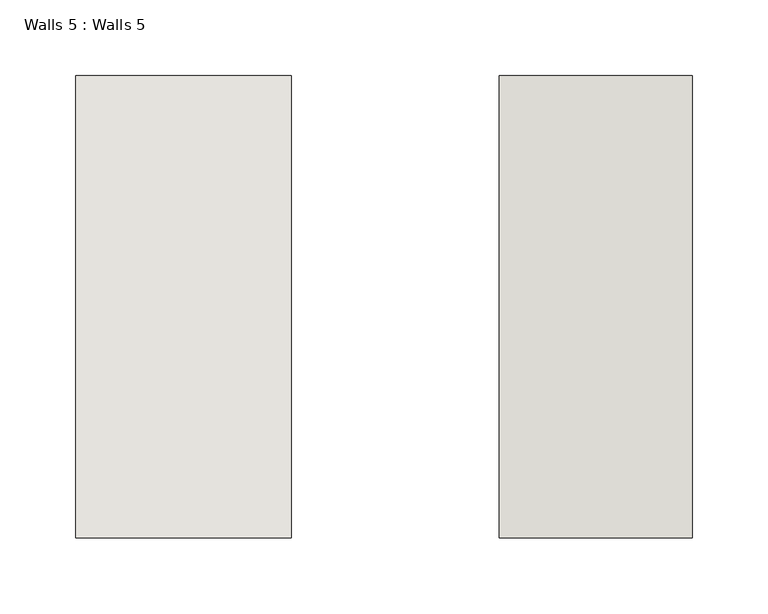
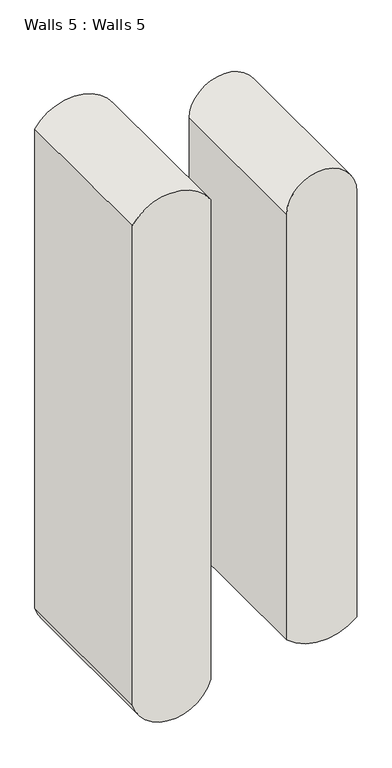
"""IFC4 building model written with IfcOpenShell, lengths in millimetres: wall geometry, Walls 5 : Walls 5."""

from ifc_helpers import new_model, si_unit, point, frame, frame_2d, origin, place, context, project, spatial, polyline, circle_curve, trimmed, segment, composite_curve, outline, extrude, source, transform, mapped, element, save


def walls_5_walls_5_0e8582f5(model_context):
    return source(origin(), model_context, "Body", "SweptSolid", [
        extrude(outline(composite_curve([segment(polyline([(1044.1671837, -3357.2945035), (127.0, -3357.2945035)]), True, "CONTINUOUS"), segment(trimmed(circle_curve(frame_2d((147.9342511, -3286.3689154)), 73.950537), [point((127.0, -3357.2945035))], [point((127.0, -3215.4433272))], False, "CARTESIAN"), True, "CONTINUOUS"), segment(polyline([(127.0, -3215.4433272), (1044.1671837, -3215.4433272)]), True, "CONTINUOUS"), segment(trimmed(circle_curve(frame_2d((996.2397239, -3286.3689154)), 85.6007036), [point((1044.1671837, -3215.4433272))], [point((1044.1671837, -3357.2945035))], False, "CARTESIAN"), True, "CONTINUOUS")], self_intersect=False)), frame((0.0, -3748.3510925, 0.0), z_axis=(0.0, 1.0, 0.0), x_axis=(0.0, 0.0, 1.0)), (0.0, 0.0, 1.0), 304.8),
        extrude(outline(composite_curve([segment(polyline([(966.6038696, -3078.1550887), (153.8038696, -3078.1550887)]), True, "CONTINUOUS"), segment(trimmed(circle_curve(frame_2d((225.1761374, -3014.6550887)), 95.5314116), [point((153.8038696, -3078.1550887))], [point((153.8038696, -2951.1550887))], False, "CARTESIAN"), True, "CONTINUOUS"), segment(polyline([(153.8038696, -2951.1550887), (966.6038696, -2951.1550887)]), True, "CONTINUOUS"), segment(trimmed(circle_curve(frame_2d((966.6038696, -3014.6550887)), 63.5), [point((966.6038696, -2951.1550887))], [point((966.6038696, -3078.1550887))], False, "CARTESIAN"), True, "CONTINUOUS")], self_intersect=False)), frame((0.0, -3748.3510925, 0.0), z_axis=(0.0, 1.0, 0.0), x_axis=(0.0, 0.0, 1.0)), (0.0, 0.0, 1.0), 304.8),
    ])


if __name__ == "__main__":
    model = new_model("IFC4")
    model_context = context("Model", 3, world=origin())
    ifc_project = project(units=[si_unit("LENGTHUNIT", "METRE", prefix="MILLI")], contexts=[model_context])
    site = spatial("IfcSite", under=ifc_project)
    building = spatial("IfcBuilding", under=site)
    placement = place(None, origin())
    walls_5_walls_5_shape = walls_5_walls_5_0e8582f5(model_context)
    element("IfcWall", 1, ObjectType="Walls 5 : Walls 5", at=placement, inside=building, context=model_context, shape_type="MappedRepresentation", body=[
        mapped(walls_5_walls_5_shape, transform((0.0, 0.0, 0.0), x_axis=(1.0, 0.0, 0.0), y_axis=(0.0, 1.0, 0.0), z_axis=(0.0, 0.0, 1.0))),
    ])
    save(model, "model.ifc")

# Revit data of these elements
# Element 1 (IfcWall, "Walls 5 : Walls 5")
#   Materials on its faces: "Default Wall"
# Materials
#   "Default Wall": colour RGB 80 80 80, transparency 0
